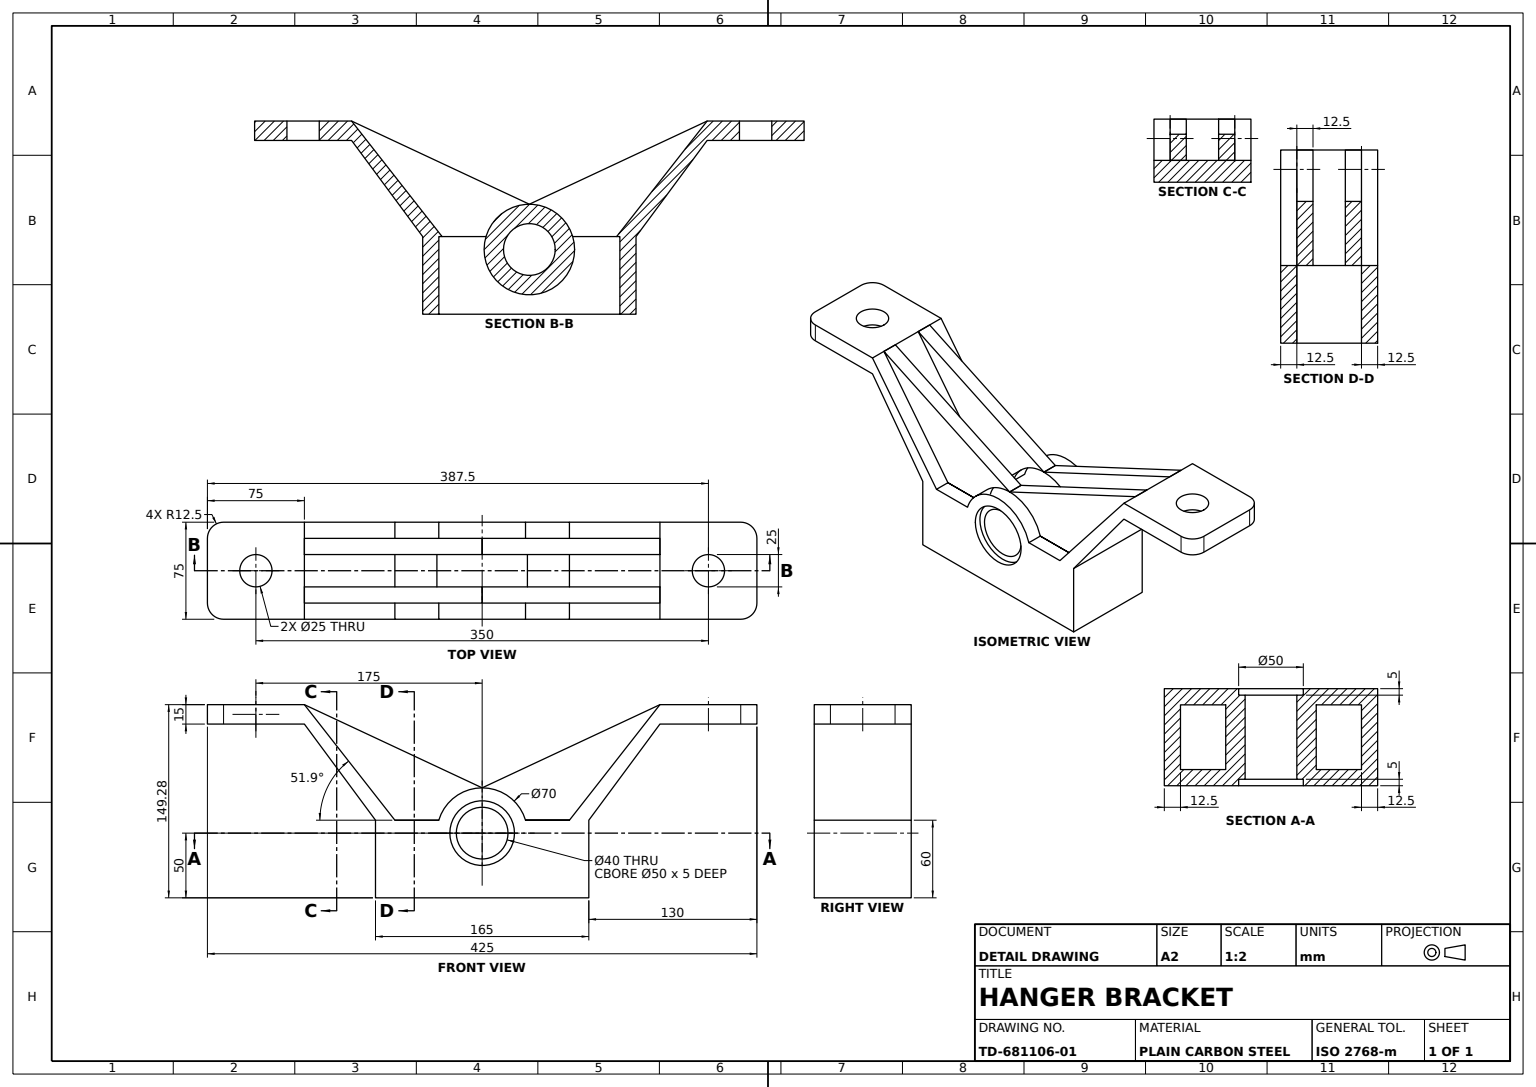
from build123d import *

# Parameters (mm, degrees)
BRACKET_BODY_THIN_60X12_5_DEPTH = 60
MOUNTING_FLANGE_PADS_DEPTH      = 75
FLANGE_HOLES_SKETCH_R           = 12.5
FLANGE_MOUNTING_HOLES_2X_DEPTH  = 75
FLANGE_CORNER_FILLET_R12_5_A_R  = 12.5
FLANGE_CORNER_FILLET_R12_5_B_R  = 12.5
BEARING_BOSS_SKETCH_R           = 35
BEARING_BOSS_DEPTH              = 75
BORE_RECESS_A_SKETCH_R          = 25
BORE_RECESS_A_5MM_DEPTH         = 5
BEARING_BORE_SKETCH_R           = 20
BEARING_BORE_DEPTH              = 109
BORE_START                      = -5
BORE_RECESS_B_SKETCH_R          = 25
BORE_RECESS_B_5MM_DEPTH         = 5
RIB_DEPTH                       = 12.5


with BuildPart() as part:
    # Bracket Profile Sketch → Bracket Body Thin 60x12.5 (new body)
    with BuildSketch(Plane(origin=(0, 0, 0), x_dir=(1, 0, 0), z_dir=(0, 1, 0))):
        Polygon((82.5, 0), (82.5, 37.5), (-82.5, 37.5), (-82.5, -37.5), (82.5, -37.5), align=None)
        Polygon((70, 0), (70, 25), (-70, 25), (-70, -25), (70, -25), align=None, mode=Mode.SUBTRACT)
    extrude(amount=BRACKET_BODY_THIN_60X12_5_DEPTH)

    # Flange Pads Sketch → Mounting Flange Pads (add)
    with BuildSketch(Plane.XY.offset(37.5)):
        Polygon((82.5, 60), (67.5, 60), (137.5, 149.280992191), (212.5, 149.280992191), (212.5, 134.280992191), (137.5, 134.280992191), align=None)
        Polygon((-137.5, 149.280992191), (-67.5, 60), (-82.5, 60), (-137.5, 134.280992191), (-212.5, 134.280992191), (-212.5, 149.280992191), align=None)
    extrude(amount=-MOUNTING_FLANGE_PADS_DEPTH)

    # Flange Holes Sketch → Flange Mounting Holes 2x (cut)
    with BuildSketch(Plane(origin=(0, 149.280992191, 0), x_dir=(1, 0, 0), z_dir=(0, 1, 0))):
        with Locations(Location((175, 0, 0), (0, 0, 180))):
            Circle(FLANGE_HOLES_SKETCH_R)
        with Locations(Location((-175, 0, 0), (0, 0, 180))):
            Circle(FLANGE_HOLES_SKETCH_R)
    extrude(amount=-FLANGE_MOUNTING_HOLES_2X_DEPTH, mode=Mode.SUBTRACT)

    # Flange Corner Fillet R12.5 A
    flange_corner_fillet_r12_5_a_edges = [part.edges().sort_by_distance(p)[0] for p in [
        (-212.5, 141.780992191, 37.5),
        (212.5, 141.780992191, 37.5),
    ]]
    fillet(flange_corner_fillet_r12_5_a_edges, radius=FLANGE_CORNER_FILLET_R12_5_A_R)

    # Flange Corner Fillet R12.5 B
    flange_corner_fillet_r12_5_b_edges = [part.edges().sort_by_distance(p)[0] for p in [
        (-212.5, 141.780992191, -37.5),
        (212.5, 141.780992191, -37.5),
    ]]
    fillet(flange_corner_fillet_r12_5_b_edges, radius=FLANGE_CORNER_FILLET_R12_5_B_R)

    # Bearing Boss Sketch → Bearing Boss (add)
    with BuildSketch(Plane.XY.offset(37.5)):
        with Locations(Location((0, 50, 0), (0, 0, 16.601549599))):
            Circle(BEARING_BOSS_SKETCH_R)
    extrude(amount=-BEARING_BOSS_DEPTH)

    # Bore Recess A Sketch → Bore Recess A 5mm (cut)
    with BuildSketch(Plane.XY.offset(37.5)):
        with Locations((0, 50)):
            Circle(BORE_RECESS_A_SKETCH_R)
    extrude(amount=-BORE_RECESS_A_5MM_DEPTH, mode=Mode.SUBTRACT)

    # Bearing Bore Sketch → Bearing Bore (cut)
    with BuildSketch(Plane.XY.offset(32.5)):
        with Locations((0, 50)):
            Circle(BEARING_BORE_SKETCH_R)
    extrude(amount=-BEARING_BORE_DEPTH, mode=Mode.SUBTRACT)

    # Bore Recess B Sketch → Bore Recess B 5mm (cut)
    with BuildSketch(Plane(origin=(0, 0, -37.5), x_dir=(-1, 0, 0), z_dir=(0, 0, -1)).offset(BORE_START)):
        with Locations(Location((0, 50, 0), (0, 0, 180))):
            Circle(BORE_RECESS_B_SKETCH_R)
    extrude(amount=BORE_RECESS_B_5MM_DEPTH, mode=Mode.SUBTRACT)


with BuildPart() as body_2:
    # Rib Sketch → Rib (new body)
    with BuildSketch(Plane.XY.offset(25)):
        with BuildLine():
            Line((-137.5, 149.280992191), (0, 85))
            ThreePointArc((0, 85), (-20.916500663, 78.062430401), (-33.541019662, 60))
            Line((-33.541019662, 60), (-67.5, 60))
            Line((-67.5, 60), (-137.5, 149.280992191))
        make_face()
    extrude(amount=-RIB_DEPTH)


with BuildPart() as body_3:
    # Rib Mirror Front Plane: mirrored copy
    add(body_2.part.mirror(Plane.XY))


with BuildPart() as body_4:
    # Rib Mirror Right Plane: mirrored copy
    add(body_3.part.mirror(Plane(origin=(0, 0, 0), x_dir=(0, 0, 1), z_dir=(1, 0, 0))))


with BuildPart() as body_5:
    # Rib Mirror Right Plane 2: mirrored copy
    add(body_2.part.mirror(Plane(origin=(0, 0, 0), x_dir=(0, 0, 1), z_dir=(1, 0, 0))))


solid = Compound([part.part, body_2.part, body_3.part, body_4.part, body_5.part])
